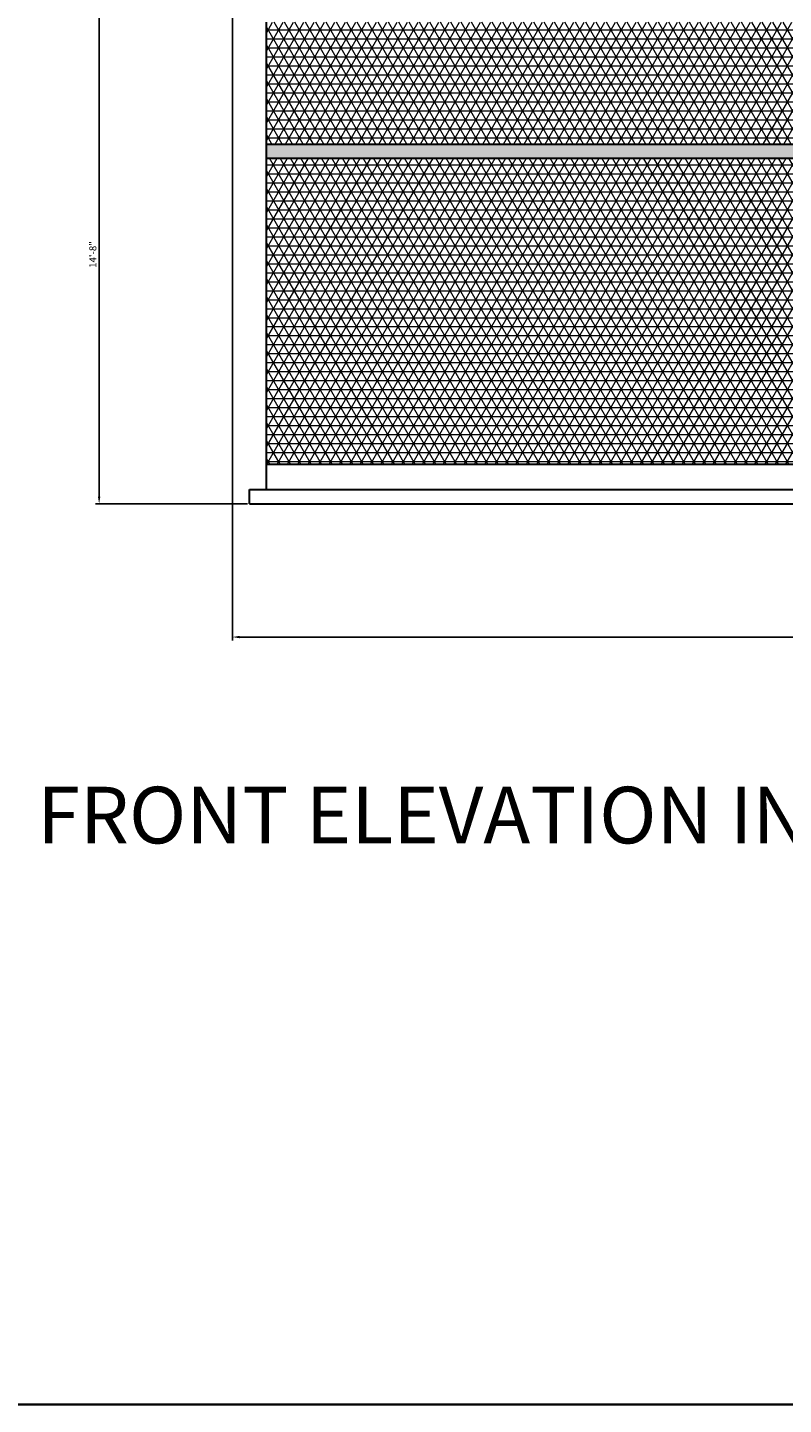
# Model space of a CAD drawing. Units: inches. Extents: x 2391 to 16591, y 7259 to 10239.
# Tile 3 of 27: x 2941 to 3208, y 7259 to 7745. Entities that reach past the tile are written whole.
import ezdxf

# ---------------------------------------------------------------- set-up
doc = ezdxf.new("R2010")
doc.units = ezdxf.units.IN
for name, color, linetype, lineweight in [('A-ANNO-DIMS', 4, 'Continuous', 18), ('A-ANNO-TITL', 3, 'Continuous', 30), ('A-ANNO-TTLB', 7, 'Continuous', 35), ('A-ELEV', 7, 'Continuous', 30), ('A-ELEV-PATT', 8, 'Continuous', 13), ('A-ELEV-SURF-PATT', 253, 'Continuous', 13)]:
    doc.layers.add(name, color=color, linetype=linetype, lineweight=lineweight)
doc.styles.get("Standard").update_dxf_attribs({"font": 'arial.ttf'})
doc.dimstyles.new('ISO-25', dxfattribs={"dimtxt": 2.5, "dimasz": 2.5, "dimexe": 1.25, "dimexo": 0.625, "dimtad": 1, "dimdec": 0, "dimlunit": 3, "dimtxsty": 'Standard', "dimcen": 2.5, "dimadec": 0, "dimazin": 0, "dimtfac": 1, "dimtdec": 0, "dimtmove": 0, "dimatfit": 3, "dimfxl": 1, "dimarcsym": 0})

# ---------------------------------------------------------------- blocks, each defined once
blk = doc.blocks.new('*D83')
at = {"layer": 'A-ANNO-DIMS', "color": 0, "lineweight": -2, "transparency": 16777216}
for p, q in [((3013.78, 7751.89), (3013.78, 7528.22)), ((3469.78, 7751.89), (3469.78, 7528.22)), ((3016.28, 7529.47), (3467.28, 7529.47))]:
    blk.add_line(p, q, dxfattribs=at)
at = {"layer": 'A-ANNO-DIMS', "color": 0, "transparency": 16777216}
for points in [[(3016.28, 7529.89), (3016.28, 7529.05), (3013.78, 7529.47)], [(3467.28, 7529.89), (3467.28, 7529.05), (3469.78, 7529.47)]]:
    blk.add_solid(points, dxfattribs=at)
at = {"layer": 'Defpoints', "color": 0, "transparency": 16777216}
for p in [(3013.78, 7752.52), (3469.78, 7752.52), (3469.78, 7529.47)]:
    blk.add_point(p, dxfattribs=at)
at = {"layer": 'A-ANNO-DIMS', "color": 0, "transparency": 16777216, "insert": (3241.78, 7531.37), "char_height": 2.5, "attachment_point": 5}
blk.add_mtext('38\'-0"', dxfattribs=at)
blk = doc.blocks.new('*D85')
at = {"layer": 'A-ANNO-DIMS', "color": 0, "lineweight": -2, "transparency": 16777216}
for p, q in [((3013.15, 7752.52), (2965.48, 7752.52)), ((2966.73, 7579.02), (2966.73, 7750.02)), ((3019.15, 7576.52), (2965.48, 7576.52))]:
    blk.add_line(p, q, dxfattribs=at)
at = {"layer": 'A-ANNO-DIMS', "color": 0, "transparency": 16777216}
for points in [[(2966.31, 7750.02), (2967.14, 7750.02), (2966.73, 7752.52)], [(2966.31, 7579.02), (2967.14, 7579.02), (2966.73, 7576.52)]]:
    blk.add_solid(points, dxfattribs=at)
at = {"layer": 'Defpoints', "color": 0, "transparency": 16777216}
for p in [(2966.73, 7752.52), (3013.78, 7752.52), (3019.78, 7576.52)]:
    blk.add_point(p, dxfattribs=at)
at = {"layer": 'A-ANNO-DIMS', "color": 0, "transparency": 16777216, "insert": (2964.83, 7664.52), "char_height": 2.5, "attachment_point": 5, "rotation": 90}
blk.add_mtext('14\'-8"', dxfattribs=at)

msp = doc.modelspace()

# ---------------------------------------------------------------- hatches: boundary and pattern name
at = {"layer": 'A-ELEV-PATT'}
h = msp.add_hatch(dxfattribs=at)
h.set_pattern_fill('NET3', color=256)
h.paths.add_polyline_path([(3457.78, 8232.52), (3339.28, 8232.52), (3339.28, 8076.52), (3457.78, 8076.52)])
h.paths.add_polyline_path([(3415.03, 8124.52), (3373.03, 8124.52), (3373.03, 8178.52), (3415.03, 8178.52)], flags=16)
h.paths.add_polyline_path([(3412.03, 8127.52), (3376.03, 8127.52), (3376.03, 8175.52), (3412.03, 8175.52)], flags=0)
h.paths.add_polyline_path([(3457.78, 8070.52), (3339.28, 8070.52), (3339.28, 7914.52), (3457.78, 7914.52)])
h.paths.add_polyline_path([(3415.03, 7962.52), (3373.03, 7962.52), (3373.03, 8016.52), (3415.03, 8016.52)], flags=16)
h.paths.add_polyline_path([(3412.03, 7965.52), (3376.03, 7965.52), (3376.03, 8013.52), (3412.03, 8013.52)], flags=0)
h.paths.add_polyline_path([(3457.78, 7908.52), (3339.28, 7908.52), (3339.28, 7752.52), (3457.78, 7752.52)])
h.paths.add_polyline_path([(3415.03, 7800.52), (3373.03, 7800.52), (3373.03, 7854.52), (3415.03, 7854.52)], flags=16)
h.paths.add_polyline_path([(3412.03, 7803.52), (3376.03, 7803.52), (3376.03, 7851.52), (3412.03, 7851.52)], flags=0)
h.paths.add_polyline_path([(3339.28, 8232.52), (3227.28, 8232.52), (3227.28, 8076.52), (3339.28, 8076.52)])
h.paths.add_polyline_path([(3260.28, 8124.52), (3260.28, 8178.52), (3302.28, 8178.52), (3302.28, 8124.52)], flags=16)
h.paths.add_polyline_path([(3263.28, 8127.52), (3263.28, 8175.52), (3299.28, 8175.52), (3299.28, 8127.52)], flags=0)
h.paths.add_polyline_path([(3339.28, 8070.52), (3227.28, 8070.52), (3227.28, 7914.52), (3339.28, 7914.52)])
h.paths.add_polyline_path([(3260.28, 8016.52), (3302.28, 8016.52), (3302.28, 7962.52), (3260.28, 7962.52)], flags=16)
h.paths.add_polyline_path([(3263.28, 8013.52), (3299.28, 8013.52), (3299.28, 7965.52), (3263.28, 7965.52)], flags=0)
h.paths.add_polyline_path([(3339.28, 7908.52), (3227.28, 7908.52), (3227.28, 7752.52), (3339.28, 7752.52)])
h.paths.add_polyline_path([(3260.28, 7854.52), (3302.28, 7854.52), (3302.28, 7800.52), (3260.28, 7800.52)], flags=16)
h.paths.add_polyline_path([(3263.28, 7851.52), (3299.28, 7851.52), (3299.28, 7803.52), (3263.28, 7803.52)], flags=0)
h.paths.add_polyline_path([(3213.78, 7717.52), (3232.78, 7717.52), (3232.78, 7712.52), (3227.78, 7712.52), (3227.78, 7683.36), (3230.28, 7683.36), (3230.28, 7685.36), (3232.78, 7685.36), (3232.78, 7710.52), (3301.78, 7710.52), (3301.78, 7595.52), (3232.78, 7595.52), (3232.78, 7590.52), (3371.78, 7590.52), (3371.78, 7595.52), (3302.78, 7595.52), (3302.78, 7710.52), (3371.78, 7710.52), (3371.78, 7685.36), (3374.28, 7685.36), (3374.28, 7683.36), (3376.78, 7683.36), (3376.78, 7712.52), (3371.78, 7712.52), (3371.78, 7717.52), (3390.78, 7717.52), (3390.78, 7712.52), (3385.78, 7712.52), (3385.78, 7703.52), (3457.78, 7703.52), (3457.78, 7746.52), (3025.78, 7746.52), (3025.78, 7703.52), (3218.78, 7703.52), (3218.78, 7712.52), (3213.78, 7712.52)])
h.paths.add_polyline_path([(3232.78, 7679.36), (3230.28, 7679.36), (3230.28, 7681.36), (3227.78, 7681.36), (3227.78, 7623.23), (3230.28, 7623.23), (3230.28, 7625.23), (3232.78, 7625.23)], flags=17)
h.paths.add_polyline_path([(3232.78, 7619.23), (3230.28, 7619.23), (3230.28, 7621.23), (3227.78, 7621.23), (3227.78, 7590.52), (3232.78, 7590.52)], flags=17)
h.paths.add_polyline_path([(3376.78, 7681.36), (3374.28, 7681.36), (3374.28, 7679.36), (3371.78, 7679.36), (3371.78, 7625.23), (3374.28, 7625.23), (3374.28, 7623.23), (3376.78, 7623.23)], flags=17)
h.paths.add_polyline_path([(3376.78, 7621.23), (3374.28, 7621.23), (3374.28, 7619.23), (3371.78, 7619.23), (3371.78, 7590.52), (3376.78, 7590.52)], flags=17)
h = msp.add_hatch(dxfattribs=at)
h.set_pattern_fill('NET3', color=256)
h.paths.add_polyline_path([(3218.78, 7590.52), (3218.78, 7698.52), (3025.78, 7698.52), (3025.78, 7590.52)])
h.paths.add_polyline_path([(3457.78, 7698.52), (3385.78, 7698.52), (3385.78, 7590.52), (3457.78, 7590.52)])
at = {"layer": 'A-ELEV-SURF-PATT'}
h = msp.add_hatch(color=256, dxfattribs=at)
h.dxf.hatch_style = 1
h.paths.add_polyline_path([(3218.78, 7698.52), (3218.78, 7703.52), (3025.78, 7703.52), (3025.78, 7698.52)])
h.paths.add_polyline_path([(3213.78, 7717.52), (3213.78, 7712.52), (3232.78, 7712.52), (3232.78, 7717.52)])
h.paths.add_polyline_path([(3371.78, 7717.52), (3371.78, 7712.52), (3390.78, 7712.52), (3390.78, 7717.52)])
h.paths.add_polyline_path([(3385.78, 7703.52), (3385.78, 7698.52), (3457.78, 7698.52), (3457.78, 7703.52)])

# ---------------------------------------------------------------- linework, layer by layer
at = {"layer": 'A-ANNO-TTLB'}
msp.add_lwpolyline([(2391.28, 10239.38), (4154.2, 10239.38), (4154.2, 7258.54), (2391.28, 7258.54)], close=True, dxfattribs=at)
at = {"layer": 'A-ELEV'}
for p, q in [((3025.78, 7581.52), (3025.78, 7746.52)), ((3025.78, 7703.52), (3218.78, 7703.52)), ((3025.78, 7698.52), (3218.78, 7698.52)), ((3025.78, 7590.52), (3457.78, 7590.52)), ((3019.78, 7576.52), (3019.78, 7581.52)), ((3019.78, 7581.52), (3463.78, 7581.52)), ((3019.78, 7576.52), (3463.78, 7576.52))]:
    msp.add_line(p, q, dxfattribs=at)

# ---------------------------------------------------------------- texts
at = {"layer": 'A-ANNO-TITL', "insert": (2944.88, 7476.61), "char_height": 20, "attachment_point": 1}
msp.add_mtext_dynamic_manual_height_columns('FRONT ELEVATION IN DIFFERNT COLOR', width=1534.7599, gutter_width=12.5, heights=[0], dxfattribs=at)

# ---------------------------------------------------------------- dimensions: what is measured, and where the dimension line sits
at = {"layer": 'A-ANNO-DIMS'}
dim = msp.add_linear_dim(base=(2966.73, 7752.52), p1=(3019.78, 7576.52), p2=(3013.78, 7752.52), angle=90, dimstyle='ISO-25', override={"dimdec": 1, "dimlfac": 1, "dimrnd": 0, "dimzin": 1, "dimdsep": 46, "dimlunit": 4, "dimfrac": 2}, dxfattribs=at)
dim.commit()
dim.dimension.update_dxf_attribs({"geometry": '*D85', "text_midpoint": (2964.83, 7664.52)})
dim = msp.add_linear_dim(base=(3469.78, 7529.47), p1=(3013.78, 7752.52), p2=(3469.78, 7752.52), dimstyle='ISO-25', override={"dimdec": 1, "dimlfac": 1, "dimrnd": 0, "dimzin": 1, "dimdsep": 46, "dimlunit": 4, "dimfrac": 2}, dxfattribs=at)
dim.commit()
dim.dimension.update_dxf_attribs({"geometry": '*D83', "text_midpoint": (3241.78, 7531.37)})

doc.saveas('drawing.dxf')
